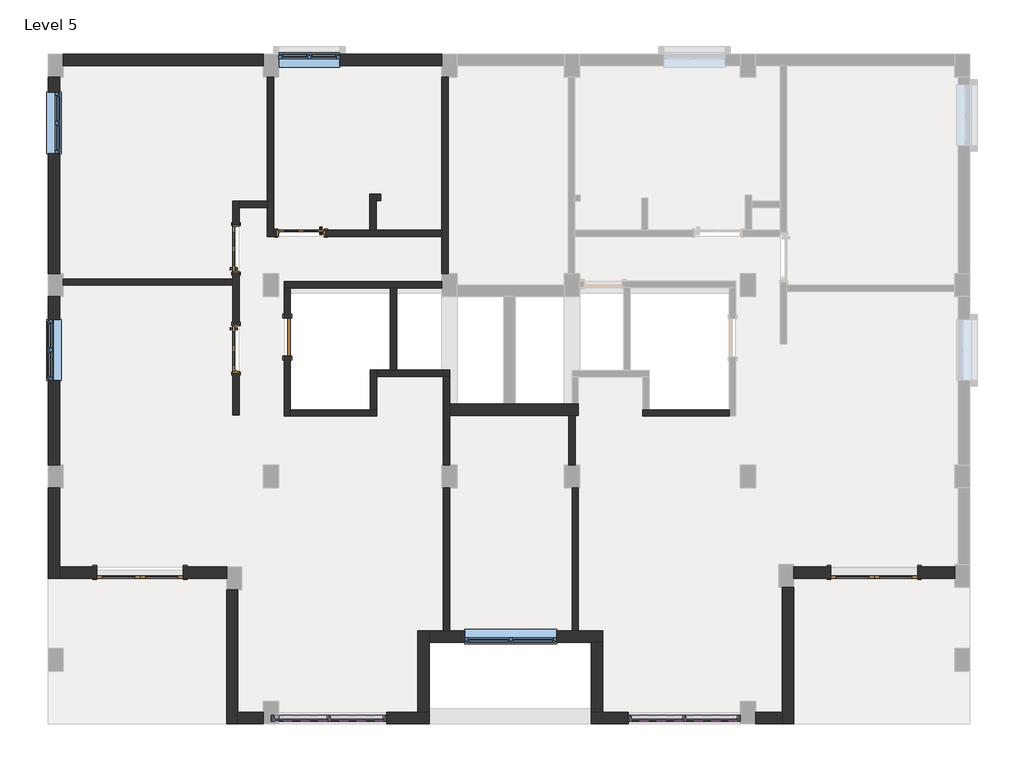
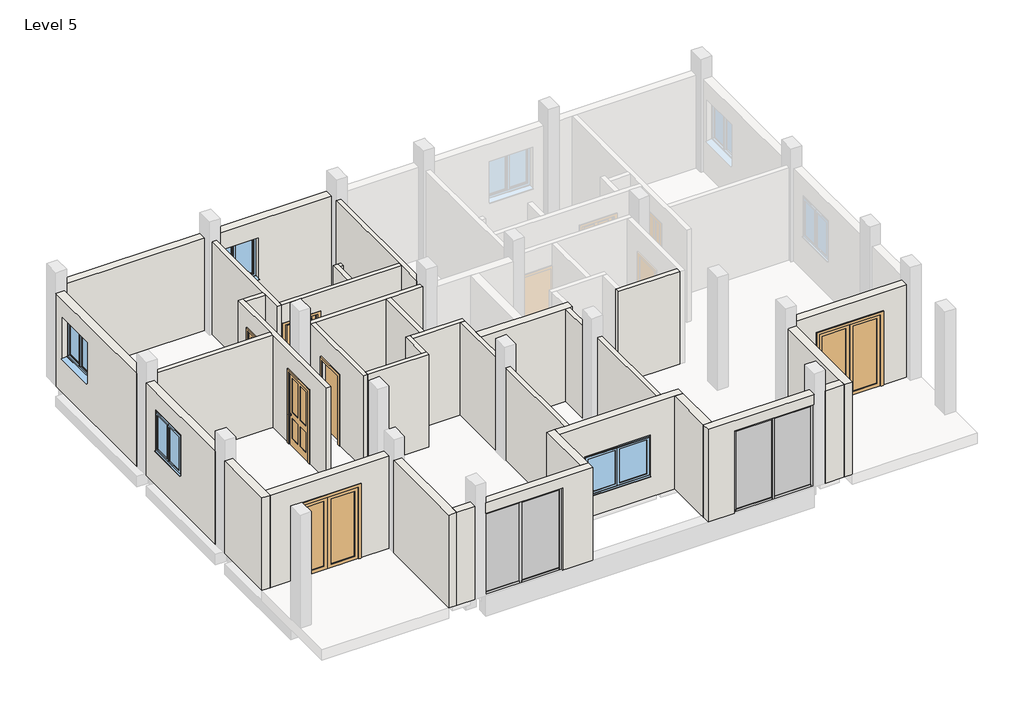
# One storey, part 1 of 3: 36 walls, 14 members, 6 doors, 4 plates, 4 windows.
"""IFC4 building model written with IfcOpenShell, lengths in millimetres."""

from ifc_helpers import new_model, si_unit, frame, origin, place, context, project, spatial, polyline, outline, extrude, faceted_brep, transform, mapped, element, save
from components import door_e52a3823, door_68a706ac, door_a823658d, door_1fe7f57d, member_a1c24a98, member_7fa39cca, member_f0fea5a5, member_ee409385, system_panel_glazed_8311221f, system_panel_glazed_a93c8db9, w2_0001_windows_4_x_4_9dec5fc7, w2_0001_window_4_x_6_83c3b52c

model = new_model("IFC4")

# Units and contexts
model_context = context("Model", 3, world=origin())
ifc_project = project(units=[si_unit("LENGTHUNIT", "METRE", prefix="MILLI")], contexts=[model_context])

# Site, building, storey
site = spatial("IfcSite", under=ifc_project)
building = spatial("IfcBuilding", under=site)
storey = spatial("IfcBuildingStorey", under=building, Name="Level 5", Elevation=6400.8)

# Doors
placement = place(None, origin())
door_shape = door_e52a3823(model_context)
element("IfcDoor", 1, ObjectType="Door-Double-Glass : 68\" x 84\"", at=placement, inside=storey, context=model_context, shape_type="MappedRepresentation", body=[
    mapped(door_shape, transform((-7309.9981098, -11554.5807833, 6400.8), x_axis=(-1.0, 0.0, 0.0), y_axis=(0.0, -1.0, 0.0), z_axis=(0.0, 0.0, 1.0))),
])
element("IfcDoor", 2, ObjectType="Door-Double-Glass : 68\" x 84\"", at=placement, inside=storey, context=model_context, shape_type="MappedRepresentation", body=[
    mapped(door_shape, transform((7313.6824202, -11554.5807833, 6400.8), x_axis=(-1.0, 0.0, 0.0), y_axis=(0.0, -1.0, 0.0), z_axis=(0.0, 0.0, 1.0))),
])
door_2_shape = door_68a706ac(model_context)
element("IfcDoor", 3, ObjectType="Door-Interior-Single-4_Panel-Wood : 36\" x 84\"", at=placement, inside=storey, context=model_context, shape_type="MappedRepresentation", body=[
    mapped(door_2_shape, transform((-5402.1925798, -5105.3620333, 6400.8), x_axis=(0.0, 1.0, 0.0), y_axis=(-1.0, 0.0, 0.0), z_axis=(0.0, 0.0, 1.0))),
])
door_3_shape = door_a823658d(model_context)
element("IfcDoor", 4, ObjectType="Door-Interior-Single-4_Panel-Wood : 36\" x 84\"", at=placement, inside=storey, context=model_context, shape_type="MappedRepresentation", body=[
    mapped(door_3_shape, transform((-4103.6175798, -4789.1311634, 6400.8), x_axis=(-1.0, 0.0, 0.0), y_axis=(0.0, -1.0, 0.0), z_axis=(0.0, 0.0, 1.0))),
])
element("IfcDoor", 5, ObjectType="Door-Interior-Single-4_Panel-Wood : 36\" x 84\"", at=placement, inside=storey, context=model_context, shape_type="MappedRepresentation", body=[
    mapped(door_3_shape, transform((-5402.1925798, -7092.9120333, 6400.8), x_axis=(0.0, -1.0, 0.0), y_axis=(1.0, 0.0, 0.0), z_axis=(0.0, 0.0, 1.0))),
])
door_4_shape = door_1fe7f57d(model_context)
element("IfcDoor", 6, ObjectType="Single-Flush : 30\" x 80\"", at=placement, inside=storey, context=model_context, shape_type="MappedRepresentation", body=[
    mapped(door_4_shape, transform((-4379.0950401, -6863.7942903, 6400.8), x_axis=(0.0, -1.0, 0.0), y_axis=(1.0, 0.0, 0.0), z_axis=(0.0, 0.0, 1.0))),
])

# Members
member_shape = member_a1c24a98(model_context)
element("IfcMember", 7, ObjectType="Rectangular Mullion : 2.5\" x 5\" rectangular", at=placement, inside=storey, context=model_context, shape_type="MappedRepresentation", body=[
    mapped(member_shape, transform((2474.9824202, -14462.5402089, 8839.2), x_axis=(0.0, 0.0, 1.0), y_axis=(0.0, 1.0, 0.0), z_axis=(-1.0, 0.0, 0.0))),
])
element("IfcMember", 8, ObjectType="Rectangular Mullion : 2.5\" x 5\" rectangular", at=placement, inside=storey, context=model_context, shape_type="MappedRepresentation", body=[
    mapped(member_shape, transform((3560.8324202, -14462.5402089, 8839.2), x_axis=(0.0, 0.0, 1.0), y_axis=(0.0, 1.0, 0.0), z_axis=(-1.0, 0.0, 0.0))),
])
element("IfcMember", 9, ObjectType="Rectangular Mullion : 2.5\" x 5\" rectangular", at=placement, inside=storey, context=model_context, shape_type="MappedRepresentation", body=[
    mapped(member_shape, transform((4583.1824202, -14462.5402089, 6400.8), x_axis=(0.0, 0.0, -1.0), y_axis=(0.0, 1.0, 0.0), z_axis=(1.0, 0.0, 0.0))),
])
element("IfcMember", 10, ObjectType="Rectangular Mullion : 2.5\" x 5\" rectangular", at=placement, inside=storey, context=model_context, shape_type="MappedRepresentation", body=[
    mapped(member_shape, transform((3497.3324202, -14462.5402089, 6400.8), x_axis=(0.0, 0.0, -1.0), y_axis=(0.0, 1.0, 0.0), z_axis=(1.0, 0.0, 0.0))),
])
member_2_shape = member_7fa39cca(model_context)
element("IfcMember", 11, ObjectType="Rectangular Mullion : 2.5\" x 5\" rectangular", at=placement, inside=storey, context=model_context, shape_type="MappedRepresentation", body=[
    mapped(member_2_shape, transform((-4637.0175798, -14462.5402089, 8839.2), x_axis=(0.0, 0.0, 1.0), y_axis=(0.0, 1.0, 0.0), z_axis=(-1.0, 0.0, 0.0))),
])
element("IfcMember", 12, ObjectType="Rectangular Mullion : 2.5\" x 5\" rectangular", at=placement, inside=storey, context=model_context, shape_type="MappedRepresentation", body=[
    mapped(member_2_shape, transform((-3519.4175798, -14462.5402089, 8839.2), x_axis=(0.0, 0.0, 1.0), y_axis=(0.0, 1.0, 0.0), z_axis=(-1.0, 0.0, 0.0))),
])
element("IfcMember", 13, ObjectType="Rectangular Mullion : 2.5\" x 5\" rectangular", at=placement, inside=storey, context=model_context, shape_type="MappedRepresentation", body=[
    mapped(member_2_shape, transform((-2465.3175798, -14462.5402089, 6400.8), x_axis=(0.0, 0.0, -1.0), y_axis=(0.0, 1.0, 0.0), z_axis=(1.0, 0.0, 0.0))),
])
element("IfcMember", 14, ObjectType="Rectangular Mullion : 2.5\" x 5\" rectangular", at=placement, inside=storey, context=model_context, shape_type="MappedRepresentation", body=[
    mapped(member_2_shape, transform((-3582.9175798, -14462.5402089, 6400.8), x_axis=(0.0, 0.0, -1.0), y_axis=(0.0, 1.0, 0.0), z_axis=(1.0, 0.0, 0.0))),
])
member_3_shape = member_f0fea5a5(model_context)
element("IfcMember", 15, ObjectType="Rectangular Mullion : 2.5\" x 5\" rectangular", at=placement, inside=storey, context=model_context, shape_type="MappedRepresentation", body=[
    mapped(member_3_shape, transform((3529.0824202, -14462.5402089, 6400.8), x_axis=(-1.0, 0.0, 0.0), y_axis=(0.0, 1.0, 0.0), z_axis=(0.0, 0.0, -1.0))),
])
element("IfcMember", 16, ObjectType="Rectangular Mullion : 2.5\" x 5\" rectangular", at=placement, inside=storey, context=model_context, shape_type="MappedRepresentation", body=[
    mapped(member_3_shape, transform((-3551.1675798, -14462.5402089, 6400.8), x_axis=(-1.0, 0.0, 0.0), y_axis=(0.0, 1.0, 0.0), z_axis=(0.0, 0.0, -1.0))),
])
member_4_shape = member_ee409385(model_context)
element("IfcMember", 17, ObjectType="Rectangular Mullion : 2.5\" x 5\" rectangular", at=placement, inside=storey, context=model_context, shape_type="MappedRepresentation", body=[
    mapped(member_4_shape, transform((2411.4824202, -14462.5402089, 6400.8), x_axis=(-1.0, 0.0, 0.0), y_axis=(0.0, 1.0, 0.0), z_axis=(0.0, 0.0, -1.0))),
])
element("IfcMember", 18, ObjectType="Rectangular Mullion : 2.5\" x 5\" rectangular", at=placement, inside=storey, context=model_context, shape_type="MappedRepresentation", body=[
    mapped(member_4_shape, transform((-4700.5175798, -14462.5402089, 6400.8), x_axis=(-1.0, 0.0, 0.0), y_axis=(0.0, 1.0, 0.0), z_axis=(0.0, 0.0, -1.0))),
])
element("IfcMember", 19, ObjectType="Rectangular Mullion : 2.5\" x 5\" rectangular", at=placement, inside=storey, context=model_context, shape_type="MappedRepresentation", body=[
    mapped(member_4_shape, transform((4646.6824202, -14462.5402089, 8839.2), x_axis=(1.0, 0.0, 0.0), y_axis=(0.0, 1.0, 0.0), z_axis=(0.0, 0.0, 1.0))),
])
element("IfcMember", 20, ObjectType="Rectangular Mullion : 2.5\" x 5\" rectangular", at=placement, inside=storey, context=model_context, shape_type="MappedRepresentation", body=[
    mapped(member_4_shape, transform((-2401.8175798, -14462.5402089, 8839.2), x_axis=(1.0, 0.0, 0.0), y_axis=(0.0, 1.0, 0.0), z_axis=(0.0, 0.0, 1.0))),
])

# Plates
system_panel_glazed_shape = system_panel_glazed_8311221f(model_context)
element("IfcPlate", 21, ObjectType="System Panel : Glazed", at=placement, inside=storey, context=model_context, shape_type="MappedRepresentation", body=[
    mapped(system_panel_glazed_shape, transform((4072.0074202, -14462.5402089, 6464.3), x_axis=(-1.0, 0.0, 0.0), y_axis=(0.0, -1.0, 0.0), z_axis=(0.0, 0.0, 1.0))),
])
element("IfcPlate", 22, ObjectType="System Panel : Glazed", at=placement, inside=storey, context=model_context, shape_type="MappedRepresentation", body=[
    mapped(system_panel_glazed_shape, transform((2986.1574202, -14462.5402089, 6464.3), x_axis=(-1.0, 0.0, 0.0), y_axis=(0.0, -1.0, 0.0), z_axis=(0.0, 0.0, 1.0))),
])
system_panel_glazed_2_shape = system_panel_glazed_a93c8db9(model_context)
element("IfcPlate", 23, ObjectType="System Panel : Glazed", at=placement, inside=storey, context=model_context, shape_type="MappedRepresentation", body=[
    mapped(system_panel_glazed_2_shape, transform((-2992.3675798, -14462.5402089, 6464.3), x_axis=(-1.0, 0.0, 0.0), y_axis=(0.0, -1.0, 0.0), z_axis=(0.0, 0.0, 1.0))),
])
element("IfcPlate", 24, ObjectType="System Panel : Glazed", at=placement, inside=storey, context=model_context, shape_type="MappedRepresentation", body=[
    mapped(system_panel_glazed_2_shape, transform((-4109.9675798, -14462.5402089, 6464.3), x_axis=(-1.0, 0.0, 0.0), y_axis=(0.0, -1.0, 0.0), z_axis=(0.0, 0.0, 1.0))),
])

# Walls
element("IfcWall", 25, ObjectType="EXTERIOR WALL 9\"", at=placement, inside=storey, context=model_context, shape_type="SweptSolid", body=[
    extrude(outline(polyline([(-4852.9175798, -1452.2061634), (-8839.9786397, -1452.2061634), (-8839.9786397, -1223.6061634), (-4852.9175798, -1223.6061634), (-4852.9175798, -1452.2061634)])), frame((0.0, 0.0, 6400.8), z_axis=(0.0, 0.0, 1.0), x_axis=(1.0, 0.0, 0.0)), (0.0, 0.0, 1.0), 2743.2),
])
element("IfcWall", 26, ObjectType="EXTERIOR WALL 9\"", at=placement, inside=storey, context=model_context, shape_type="SweptSolid", body=[
    extrude(outline(polyline([(7400.8, -3328.9175798), (7400.8, -4548.1175798), (6400.8, -4548.1175798), (6400.8, -1296.9175798), (9144.0, -1296.9175798), (9144.0, -4548.1175798), (8620.0, -4548.1175798), (8620.0, -3328.9175798), (7400.8, -3328.9175798)])), frame((0.0, -1452.2061634, 0.0), z_axis=(0.0, 1.0, 0.0), x_axis=(0.0, 0.0, 1.0)), (0.0, 0.0, 1.0), 228.6),
])
element("IfcWall", 27, ObjectType="EXTERIOR WALL 9\"", at=placement, inside=storey, context=model_context, shape_type="SweptSolid", body=[
    extrude(outline(polyline([(-1680.8061634, 6400.8), (-5600.6620333, 6400.8), (-5600.6620333, 9144.0), (-1680.8061634, 9144.0), (-1680.8061634, 6400.8)]), holes=[polyline([(-3204.8061634, 7400.8), (-1985.6061634, 7400.8), (-1985.6061634, 8620.0), (-3204.8061634, 8620.0), (-3204.8061634, 7400.8)])]), frame((-9144.7786397, 0.0, 0.0), z_axis=(1.0, 0.0, 0.0), x_axis=(0.0, 1.0, 0.0)), (0.0, 0.0, 1.0), 228.6),
])
element("IfcWall", 28, ObjectType="EXTERIOR WALL 9\"", at=placement, inside=storey, context=model_context, shape_type="SweptSolid", body=[
    extrude(outline(polyline([(-6057.8620333, 6400.8), (-9410.6620333, 6400.8), (-9410.6620333, 9144.0), (-6057.8620333, 9144.0), (-6057.8620333, 6400.8)]), holes=[polyline([(-6515.0620333, 7400.8), (-6515.0620333, 8620.0), (-7734.2620333, 8620.0), (-7734.2620333, 7400.8), (-6515.0620333, 7400.8)])]), frame((-9144.7786397, 0.0, 0.0), z_axis=(1.0, 0.0, 0.0), x_axis=(0.0, 1.0, 0.0)), (0.0, 0.0, 1.0), 228.6),
])
element("IfcWall", 29, ObjectType="EXTERIOR WALL 9\"", at=placement, inside=storey, context=model_context, shape_type="Brep", body=[
    faceted_brep([(-9144.7786397, -9867.8620333, 6400.8), (-9144.7786397, -11671.2620333, 6400.8), (-9144.7786397, -11671.2620333, 9144.0), (-9144.7786397, -9867.8620333, 9144.0), (-8916.1786397, -9867.8620333, 6400.8), (-8916.1786397, -9867.8620333, 9144.0), (-8916.1786397, -11442.6620333, 9144.0), (-8916.1786397, -11671.2620333, 9144.0), (-8916.1786397, -11671.2620333, 6400.8), (-8916.1786397, -11442.6620333, 6400.8)], [[[0, 1, 2, 3]], [[4, 5, 6, 7, 8, 9]], [[1, 0, 4, 9, 8]], [[3, 2, 7, 6, 5]], [[0, 3, 5, 4]], [[2, 1, 8, 7]]]),
])
element("IfcWall", 30, ObjectType="EXTERIOR WALL 9\"", at=placement, inside=storey, context=model_context, shape_type="SweptSolid", body=[
    extrude(outline(polyline([(9144.0, -5589.5175798), (9144.0, -8916.1786397), (6400.8, -8916.1786397), (6400.8, -8173.5981098), (8534.4, -8173.5981098), (8534.4, -6446.3981098), (6400.8, -6446.3981098), (6400.8, -5589.5175798), (9144.0, -5589.5175798)])), frame((0.0, -11671.2620333, 0.0), z_axis=(0.0, 1.0, 0.0), x_axis=(0.0, 0.0, 1.0)), (0.0, 0.0, 1.0), 228.6),
])
element("IfcWall", 31, ObjectType="EXTERIOR WALL 9\"", at=placement, inside=storey, context=model_context, shape_type="SweptSolid", body=[
    extrude(outline(polyline([(9144.0, 5713.4824202), (6400.8, 5713.4824202), (6400.8, 6450.0824202), (8534.4, 6450.0824202), (8534.4, 8177.2824202), (6400.8, 8177.2824202), (6400.8, 8913.8824202), (9144.0, 8913.8824202), (9144.0, 5713.4824202)])), frame((0.0, -11671.2620333, 0.0), z_axis=(0.0, 1.0, 0.0), x_axis=(0.0, 0.0, 1.0)), (0.0, 0.0, 1.0), 228.6),
])
element("IfcWall", 32, ObjectType="EXTERIOR WALL 9\"", at=placement, inside=storey, context=model_context, shape_type="Brep", body=[
    faceted_brep([(5484.8824202, -11849.0620333, 6400.8), (5484.8824202, -14348.2402089, 6400.8), (5484.8824202, -14576.8402089, 6400.8), (5484.8824202, -14576.8402089, 9144.0), (5484.8824202, -14348.2402089, 9144.0), (5484.8824202, -11849.0620333, 9144.0), (5713.4824202, -11849.0620333, 6400.8), (5713.4824202, -11849.0620333, 9144.0), (5713.4824202, -14576.8402089, 9144.0), (5713.4824202, -14576.8402089, 6400.8)], [[[0, 1, 2, 3, 4, 5]], [[6, 7, 8, 9]], [[2, 1, 0, 6, 9]], [[5, 4, 3, 8, 7]], [[0, 5, 7, 6]], [[3, 2, 9, 8]]]),
])
element("IfcWall", 33, ObjectType="EXTERIOR WALL 9\"", at=placement, inside=storey, context=model_context, shape_type="SweptSolid", body=[
    extrude(outline(polyline([(5484.8824202, -14576.8402089), (4951.4824202, -14576.8402089), (4951.4824202, -14348.2402089), (5484.8824202, -14348.2402089), (5484.8824202, -14576.8402089)])), frame((0.0, 0.0, 6400.8), z_axis=(0.0, 0.0, 1.0), x_axis=(1.0, 0.0, 0.0)), (0.0, 0.0, 1.0), 2743.2),
])
element("IfcWall", 34, ObjectType="EXTERIOR WALL 9\"", at=placement, inside=storey, context=model_context, shape_type="Brep", body=[
    faceted_brep([(-5589.5175798, -11899.8620333, 6400.8), (-5589.5175798, -14576.8402089, 6400.8), (-5589.5175798, -14576.8402089, 9144.0), (-5589.5175798, -11899.8620333, 9144.0), (-5360.9175798, -11899.8620333, 6400.8), (-5360.9175798, -11899.8620333, 9144.0), (-5360.9175798, -14348.2402089, 9144.0), (-5360.9175798, -14576.8402089, 9144.0), (-5360.9175798, -14576.8402089, 6400.8), (-5360.9175798, -14348.2402089, 6400.8)], [[[0, 1, 2, 3]], [[4, 5, 6, 7, 8, 9]], [[1, 0, 4, 9, 8]], [[3, 2, 7, 6, 5]], [[0, 3, 5, 4]], [[2, 1, 8, 7]]]),
])
element("IfcWall", 35, ObjectType="EXTERIOR WALL 9\"", at=placement, inside=storey, context=model_context, shape_type="SweptSolid", body=[
    extrude(outline(polyline([(-5360.9175798, -14348.2402089), (-4852.9175798, -14348.2402089), (-4852.9175798, -14576.8402089), (-5360.9175798, -14576.8402089), (-5360.9175798, -14348.2402089)])), frame((0.0, 0.0, 6400.8), z_axis=(0.0, 0.0, 1.0), x_axis=(1.0, 0.0, 0.0)), (0.0, 0.0, 1.0), 2743.2),
])
element("IfcWall", 36, ObjectType="EXTERIOR WALL 9\"", at=placement, inside=storey, context=model_context, shape_type="Brep", body=[
    faceted_brep([(1674.8824202, -14348.2402089, 9144.0), (1903.4824202, -14348.2402089, 9144.0), (4646.6824202, -14348.2402089, 9144.0), (4646.6824202, -14348.2402089, 8839.2), (2411.4824202, -14348.2402089, 8839.2), (2411.4824202, -14348.2402089, 6400.8), (1903.4824202, -14348.2402089, 6400.8), (1674.8824202, -14348.2402089, 6400.8), (4646.6824202, -14576.8402089, 9144.0), (1674.8824202, -14576.8402089, 9144.0), (1674.8824202, -14576.8402089, 6400.8), (2411.4824202, -14576.8402089, 6400.8), (2411.4824202, -14576.8402089, 8839.2), (4646.6824202, -14576.8402089, 8839.2)], [[[0, 1, 2, 3, 4, 5, 6, 7]], [[8, 9, 10, 11, 12, 13]], [[10, 7, 6, 5, 11]], [[2, 1, 0, 9, 8]], [[2, 8, 13, 3]], [[0, 7, 10, 9]], [[4, 12, 11, 5]], [[12, 4, 3, 13]]]),
])
element("IfcWall", 37, ObjectType="EXTERIOR WALL 9\"", at=placement, inside=storey, context=model_context, shape_type="Brep", body=[
    faceted_brep([(-1550.9175798, -14576.8402089, 9144.0), (-4548.1175798, -14576.8402089, 9144.0), (-4548.1175798, -14576.8402089, 8839.2), (-2401.8175798, -14576.8402089, 8839.2), (-2401.8175798, -14576.8402089, 6400.8), (-1550.9175798, -14576.8402089, 6400.8), (-4548.1175798, -14348.2402089, 9144.0), (-1779.5175798, -14348.2402089, 9144.0), (-1550.9175798, -14348.2402089, 9144.0), (-1550.9175798, -14348.2402089, 6400.8), (-1779.5175798, -14348.2402089, 6400.8), (-2401.8175798, -14348.2402089, 6400.8), (-2401.8175798, -14348.2402089, 8839.2), (-4548.1175798, -14348.2402089, 8839.2)], [[[0, 1, 2, 3, 4, 5]], [[6, 7, 8, 9, 10, 11, 12, 13]], [[9, 5, 4, 11, 10]], [[1, 0, 8, 7, 6]], [[1, 6, 13, 2]], [[0, 5, 9, 8]], [[3, 12, 11, 4]], [[12, 3, 2, 13]]]),
])
element("IfcWall", 38, ObjectType="EXTERIOR WALL 9\"", at=placement, inside=storey, context=model_context, shape_type="Brep", body=[
    faceted_brep([(-1550.9175798, -14348.2402089, 6400.8), (-1550.9175798, -12951.2402089, 6400.8), (-1550.9175798, -12722.6402089, 6400.8), (-1550.9175798, -12722.6402089, 9144.0), (-1550.9175798, -12951.2402089, 9144.0), (-1550.9175798, -14348.2402089, 9144.0), (-1779.5175798, -14348.2402089, 6400.8), (-1779.5175798, -14348.2402089, 9144.0), (-1779.5175798, -12722.6402089, 9144.0), (-1779.5175798, -12722.6402089, 6400.8)], [[[0, 1, 2, 3, 4, 5]], [[6, 7, 8, 9]], [[2, 1, 0, 6, 9]], [[5, 4, 3, 8, 7]], [[0, 5, 7, 6]], [[3, 2, 9, 8]]]),
])
element("IfcWall", 39, ObjectType="EXTERIOR WALL 9\"", at=placement, inside=storey, context=model_context, shape_type="Brep", body=[
    faceted_brep([(-1550.9175798, -12951.2402089, 6400.8), (1674.8824202, -12951.2402089, 6400.8), (1903.4824202, -12951.2402089, 6400.8), (1903.4824202, -12951.2402089, 9144.0), (1674.8824202, -12951.2402089, 9144.0), (-1550.9175798, -12951.2402089, 9144.0), (-839.7175798, -12951.2402089, 7010.4), (-839.7175798, -12951.2402089, 8229.6), (989.0824202, -12951.2402089, 8229.6), (989.0824202, -12951.2402089, 7010.4), (-1550.9175798, -12722.6402089, 6400.8), (-1550.9175798, -12722.6402089, 9144.0), (-1271.5175798, -12722.6402089, 9144.0), (-1144.5175798, -12722.6402089, 9144.0), (1293.8824202, -12722.6402089, 9144.0), (1420.8824202, -12722.6402089, 9144.0), (1903.4824202, -12722.6402089, 9144.0), (1903.4824202, -12722.6402089, 6400.8), (1420.8824202, -12722.6402089, 6400.8), (1293.8824202, -12722.6402089, 6400.8), (-1144.5175798, -12722.6402089, 6400.8), (-1271.5175798, -12722.6402089, 6400.8), (-839.7175798, -12722.6402089, 7010.4), (989.0824202, -12722.6402089, 7010.4), (989.0824202, -12722.6402089, 8229.6), (-839.7175798, -12722.6402089, 8229.6)], [[[0, 1, 2, 3, 4, 5], [6, 7, 8, 9]], [[10, 11, 12, 13, 14, 15, 16, 17, 18, 19, 20, 21], [22, 23, 24, 25]], [[2, 1, 0, 10, 21, 20, 19, 18, 17]], [[5, 4, 3, 16, 15, 14, 13, 12, 11]], [[0, 5, 11, 10]], [[3, 2, 17, 16]], [[7, 6, 22, 25]], [[8, 7, 25, 24]], [[9, 8, 24, 23]], [[6, 9, 23, 22]]]),
])
element("IfcWall", 40, ObjectType="EXTERIOR WALL 9\"", at=placement, inside=storey, context=model_context, shape_type="SweptSolid", body=[
    extrude(outline(polyline([(1674.8824202, -14348.2402089), (1674.8824202, -12951.2402089), (1903.4824202, -12951.2402089), (1903.4824202, -14348.2402089), (1674.8824202, -14348.2402089)])), frame((0.0, 0.0, 6400.8), z_axis=(0.0, 0.0, 1.0), x_axis=(1.0, 0.0, 0.0)), (0.0, 0.0, 1.0), 2743.2),
])
element("IfcWall", 41, ObjectType="EXTERIOR WALL 9\"", at=placement, inside=storey, context=model_context, shape_type="Brep", body=[
    faceted_brep([(-1144.5175798, -8426.4120333, 6400.8), (1230.3824202, -8426.4120333, 6400.8), (1357.3824202, -8426.4120333, 6400.8), (1420.8824202, -8426.4120333, 6400.8), (1420.8824202, -8426.4120333, 9144.0), (1357.3824202, -8426.4120333, 9144.0), (1230.3824202, -8426.4120333, 9144.0), (-1144.5175798, -8426.4120333, 9144.0), (-1144.5175798, -8197.8120333, 6400.8), (-1144.5175798, -8197.8120333, 9144.0), (-65.0175798, -8197.8120333, 9144.0), (163.5824202, -8197.8120333, 9144.0), (1293.8824202, -8197.8120333, 9144.0), (1420.8824202, -8197.8120333, 9144.0), (1420.8824202, -8197.8120333, 6400.8), (1293.8824202, -8197.8120333, 6400.8), (163.5824202, -8197.8120333, 6400.8), (-65.0175798, -8197.8120333, 6400.8)], [[[0, 1, 2, 3, 4, 5, 6, 7]], [[8, 9, 10, 11, 12, 13, 14, 15, 16, 17]], [[3, 2, 1, 0, 8, 17, 16, 15, 14]], [[7, 6, 5, 4, 13, 12, 11, 10, 9]], [[0, 7, 9, 8]], [[4, 3, 14, 13]]]),
])
element("IfcWall", 42, ObjectType="INTERIOR WALL 5\"", at=placement, inside=storey, context=model_context, shape_type="SweptSolid", body=[
    extrude(outline(polyline([(-5462.5175798, -5829.2620333), (-8839.9786397, -5829.2620333), (-8839.9786397, -5702.2620333), (-5462.5175798, -5702.2620333), (-5462.5175798, -5829.2620333)])), frame((0.0, 0.0, 6400.8), z_axis=(0.0, 0.0, 1.0), x_axis=(1.0, 0.0, 0.0)), (0.0, 0.0, 1.0), 2743.2),
])
element("IfcWall", 43, ObjectType="INTERIOR WALL 5\"", at=placement, inside=storey, context=model_context, shape_type="Brep", body=[
    faceted_brep([(-5462.5175798, -8420.0620333, 6400.8), (-5462.5175798, -8420.0620333, 9144.0), (-5462.5175798, -5829.2620333, 9144.0), (-5462.5175798, -5702.2620333, 9144.0), (-5462.5175798, -4153.3104011, 9144.0), (-5462.5175798, -4153.3104011, 6400.8), (-5462.5175798, -4622.7620333, 6400.8), (-5462.5175798, -4622.7620333, 8559.8), (-5462.5175798, -5587.9620333, 8559.8), (-5462.5175798, -5587.9620333, 6400.8), (-5462.5175798, -5702.2620333, 6400.8), (-5462.5175798, -5829.2620333, 6400.8), (-5462.5175798, -6610.3120333, 6400.8), (-5462.5175798, -6610.3120333, 8559.8), (-5462.5175798, -7575.5120333, 8559.8), (-5462.5175798, -7575.5120333, 6400.8), (-5335.5175798, -8420.0620333, 9144.0), (-5335.5175798, -8420.0620333, 6400.8), (-5335.5175798, -7575.5120333, 6400.8), (-5335.5175798, -7575.5120333, 8559.8), (-5335.5175798, -6610.3120333, 8559.8), (-5335.5175798, -6610.3120333, 6400.8), (-5335.5175798, -5587.9620333, 6400.8), (-5335.5175798, -5587.9620333, 8559.8), (-5335.5175798, -4622.7620333, 8559.8), (-5335.5175798, -4622.7620333, 6400.8), (-5335.5175798, -4280.3104011, 6400.8), (-5335.5175798, -4153.3104011, 6400.8), (-5335.5175798, -4153.3104011, 9144.0), (-5335.5175798, -4280.3104011, 9144.0)], [[[0, 1, 2, 3, 4, 5, 6, 7, 8, 9, 10, 11, 12, 13, 14, 15]], [[16, 17, 18, 19, 20, 21, 22, 23, 24, 25, 26, 27, 28, 29]], [[17, 0, 15, 18]], [[5, 27, 26, 25, 6]], [[9, 22, 21, 12, 11, 10]], [[1, 0, 17, 16]], [[4, 3, 2, 1, 16, 29, 28]], [[5, 4, 28, 27]], [[24, 7, 6, 25]], [[7, 24, 23, 8]], [[8, 23, 22, 9]], [[14, 19, 18, 15]], [[19, 14, 13, 20]], [[20, 13, 12, 21]]]),
])
element("IfcWall", 44, ObjectType="INTERIOR WALL 5\"", at=placement, inside=storey, context=model_context, shape_type="SweptSolid", body=[
    extrude(outline(polyline([(-4776.7175798, -4280.3104011), (-5335.5175798, -4280.3104011), (-5335.5175798, -4153.3104011), (-4776.7175798, -4153.3104011), (-4776.7175798, -4280.3104011)])), frame((0.0, 0.0, 6400.8), z_axis=(0.0, 0.0, 1.0), x_axis=(1.0, 0.0, 0.0)), (0.0, 0.0, 1.0), 2743.2),
])
element("IfcWall", 45, ObjectType="INTERIOR WALL 5\"", at=placement, inside=storey, context=model_context, shape_type="Brep", body=[
    faceted_brep([(-4776.7175798, -1680.8061634, 6400.8), (-4776.7175798, -4153.3104011, 6400.8), (-4776.7175798, -4280.3104011, 6400.8), (-4776.7175798, -4855.8061634, 6400.8), (-4776.7175798, -4855.8061634, 9144.0), (-4776.7175798, -4280.3104011, 9144.0), (-4776.7175798, -4153.3104011, 9144.0), (-4776.7175798, -1680.8061634, 9144.0), (-4649.7175798, -1680.8061634, 6400.8), (-4649.7175798, -1680.8061634, 9144.0), (-4649.7175798, -4728.8061634, 9144.0), (-4649.7175798, -4855.8061634, 9144.0), (-4649.7175798, -4855.8061634, 6400.8), (-4649.7175798, -4728.8061634, 6400.8)], [[[0, 1, 2, 3, 4, 5, 6, 7]], [[8, 9, 10, 11, 12, 13]], [[3, 2, 1, 0, 8, 13, 12]], [[7, 6, 5, 4, 11, 10, 9]], [[0, 7, 9, 8]], [[4, 3, 12, 11]]]),
])
element("IfcWall", 46, ObjectType="INTERIOR WALL 5\"", at=placement, inside=storey, context=model_context, shape_type="Brep", body=[
    faceted_brep([(-1296.9175798, -4855.8061634, 9144.0), (-4649.7175798, -4855.8061634, 9144.0), (-4649.7175798, -4855.8061634, 6400.8), (-4586.2175798, -4855.8061634, 6400.8), (-4586.2175798, -4855.8061634, 8559.8), (-3621.0175798, -4855.8061634, 8559.8), (-3621.0175798, -4855.8061634, 6400.8), (-1296.9175798, -4855.8061634, 6400.8), (-4649.7175798, -4728.8061634, 9144.0), (-2732.0175798, -4728.8061634, 9144.0), (-2605.0175798, -4728.8061634, 9144.0), (-1296.9175798, -4728.8061634, 9144.0), (-1296.9175798, -4728.8061634, 6400.8), (-2605.0175798, -4728.8061634, 6400.8), (-2732.0175798, -4728.8061634, 6400.8), (-3621.0175798, -4728.8061634, 6400.8), (-3621.0175798, -4728.8061634, 8559.8), (-4586.2175798, -4728.8061634, 8559.8), (-4586.2175798, -4728.8061634, 6400.8), (-4649.7175798, -4728.8061634, 6400.8)], [[[0, 1, 2, 3, 4, 5, 6, 7]], [[8, 9, 10, 11, 12, 13, 14, 15, 16, 17, 18, 19]], [[2, 19, 18, 3]], [[12, 7, 6, 15, 14, 13]], [[1, 0, 11, 10, 9, 8]], [[2, 1, 8, 19]], [[0, 7, 12, 11]], [[17, 4, 3, 18]], [[4, 17, 16, 5]], [[5, 16, 15, 6]]]),
])
element("IfcWall", 47, ObjectType="INTERIOR WALL 5\"", at=placement, inside=storey, context=model_context, shape_type="Brep", body=[
    faceted_brep([(-1296.9175798, -1680.8061634, 6400.8), (-1296.9175798, -4728.8061634, 6400.8), (-1296.9175798, -4855.8061634, 6400.8), (-1296.9175798, -5600.6620333, 6400.8), (-1296.9175798, -5600.6620333, 9144.0), (-1296.9175798, -4855.8061634, 9144.0), (-1296.9175798, -4728.8061634, 9144.0), (-1296.9175798, -1680.8061634, 9144.0), (-1169.9175798, -1680.8061634, 6400.8), (-1169.9175798, -1680.8061634, 9144.0), (-1169.9175798, -5600.6620333, 9144.0), (-1169.9175798, -5600.6620333, 6400.8)], [[[0, 1, 2, 3, 4, 5, 6, 7]], [[8, 9, 10, 11]], [[3, 2, 1, 0, 8, 11]], [[4, 3, 11, 10]], [[7, 6, 5, 4, 10, 9]], [[0, 7, 9, 8]]]),
])
element("IfcWall", 48, ObjectType="INTERIOR WALL 5\"", at=placement, inside=storey, context=model_context, shape_type="Brep", body=[
    faceted_brep([(-2605.0175798, -4728.8061634, 6400.8), (-2605.0175798, -4144.6061634, 6400.8), (-2605.0175798, -4017.6061634, 6400.8), (-2605.0175798, -4017.6061634, 9144.0), (-2605.0175798, -4144.6061634, 9144.0), (-2605.0175798, -4728.8061634, 9144.0), (-2732.0175798, -4728.8061634, 6400.8), (-2732.0175798, -4728.8061634, 9144.0), (-2732.0175798, -4017.6061634, 9144.0), (-2732.0175798, -4017.6061634, 6400.8)], [[[0, 1, 2, 3, 4, 5]], [[6, 7, 8, 9]], [[2, 1, 0, 6, 9]], [[5, 4, 3, 8, 7]], [[0, 5, 7, 6]], [[3, 2, 9, 8]]]),
])
element("IfcWall", 49, ObjectType="INTERIOR WALL 5\"", at=placement, inside=storey, context=model_context, shape_type="SweptSolid", body=[
    extrude(outline(polyline([(-2605.0175798, -4017.6061634), (-2516.1175798, -4017.6061634), (-2516.1175798, -4144.6061634), (-2605.0175798, -4144.6061634), (-2605.0175798, -4017.6061634)])), frame((0.0, 0.0, 6400.8), z_axis=(0.0, 0.0, 1.0), x_axis=(1.0, 0.0, 0.0)), (0.0, 0.0, 1.0), 2743.2),
])
element("IfcWall", 50, ObjectType="INTERIOR WALL 5\"", at=placement, inside=storey, context=model_context, shape_type="Brep", body=[
    faceted_brep([(-4442.5950401, -5885.8942903, 6400.8), (-4315.5950401, -5885.8942903, 6400.8), (-2325.6175798, -5885.8942903, 6400.8), (-2198.6175798, -5885.8942903, 6400.8), (-1296.9175798, -5885.8942903, 6400.8), (-1296.9175798, -5885.8942903, 9144.0), (-2198.6175798, -5885.8942903, 9144.0), (-2325.6175798, -5885.8942903, 9144.0), (-4315.5950401, -5885.8942903, 9144.0), (-4442.5950401, -5885.8942903, 9144.0), (-4442.5950401, -5758.8942903, 6400.8), (-4442.5950401, -5758.8942903, 9144.0), (-1296.9175798, -5758.8942903, 9144.0), (-1296.9175798, -5758.8942903, 6400.8)], [[[0, 1, 2, 3, 4, 5, 6, 7, 8, 9]], [[10, 11, 12, 13]], [[4, 3, 2, 1, 0, 10, 13]], [[5, 4, 13, 12]], [[9, 8, 7, 6, 5, 12, 11]], [[0, 9, 11, 10]]]),
])
element("IfcWall", 51, ObjectType="INTERIOR WALL 5\"", at=placement, inside=storey, context=model_context, shape_type="Brep", body=[
    faceted_brep([(-4442.5950401, -7244.7942903, 8432.8), (-4442.5950401, -7244.7942903, 6400.8), (-4442.5950401, -8439.1120333, 6400.8), (-4442.5950401, -8439.1120333, 9144.0), (-4442.5950401, -5885.8942903, 9144.0), (-4442.5950401, -5885.8942903, 6400.8), (-4442.5950401, -6482.7942903, 6400.8), (-4442.5950401, -6482.7942903, 8432.8), (-4315.5950401, -8439.1120333, 6400.8), (-4315.5950401, -8312.1120333, 6400.8), (-4315.5950401, -7244.7942903, 6400.8), (-4315.5950401, -7244.7942903, 8432.8), (-4315.5950401, -6482.7942903, 8432.8), (-4315.5950401, -6482.7942903, 6400.8), (-4315.5950401, -5885.8942903, 6400.8), (-4315.5950401, -5885.8942903, 9144.0), (-4315.5950401, -8312.1120333, 9144.0), (-4315.5950401, -8439.1120333, 9144.0)], [[[0, 1, 2, 3, 4, 5, 6, 7]], [[8, 9, 10, 11, 12, 13, 14, 15, 16, 17]], [[6, 5, 14, 13]], [[2, 1, 10, 9, 8]], [[4, 3, 17, 16, 15]], [[5, 4, 15, 14]], [[3, 2, 8, 17]], [[11, 10, 1, 0]], [[12, 11, 0, 7]], [[13, 12, 7, 6]]]),
])
element("IfcWall", 52, ObjectType="INTERIOR WALL 5\"", at=placement, inside=storey, context=model_context, shape_type="Brep", body=[
    faceted_brep([(-4315.5950401, -8439.1120333, 6400.8), (-2601.0950401, -8439.1120333, 6400.8), (-2601.0950401, -8439.1120333, 9144.0), (-4315.5950401, -8439.1120333, 9144.0), (-4315.5950401, -8312.1120333, 6400.8), (-4315.5950401, -8312.1120333, 9144.0), (-2728.0950401, -8312.1120333, 9144.0), (-2601.0950401, -8312.1120333, 9144.0), (-2601.0950401, -8312.1120333, 6400.8), (-2728.0950401, -8312.1120333, 6400.8)], [[[0, 1, 2, 3]], [[4, 5, 6, 7, 8, 9]], [[1, 0, 4, 9, 8]], [[3, 2, 7, 6, 5]], [[0, 3, 5, 4]], [[2, 1, 8, 7]]]),
])
element("IfcWall", 53, ObjectType="INTERIOR WALL 5\"", at=placement, inside=storey, context=model_context, shape_type="Brep", body=[
    faceted_brep([(-2601.0950401, -8312.1120333, 6400.8), (-2601.0950401, -7651.7120333, 6400.8), (-2601.0950401, -7524.7120333, 6400.8), (-2601.0950401, -7524.7120333, 9144.0), (-2601.0950401, -7651.7120333, 9144.0), (-2601.0950401, -8312.1120333, 9144.0), (-2728.0950401, -8312.1120333, 6400.8), (-2728.0950401, -8312.1120333, 9144.0), (-2728.0950401, -7524.7120333, 9144.0), (-2728.0950401, -7524.7120333, 6400.8)], [[[0, 1, 2, 3, 4, 5]], [[6, 7, 8, 9]], [[2, 1, 0, 6, 9]], [[5, 4, 3, 8, 7]], [[0, 5, 7, 6]], [[3, 2, 9, 8]]]),
])
element("IfcWall", 54, ObjectType="INTERIOR WALL 5\"", at=placement, inside=storey, context=model_context, shape_type="Brep", body=[
    faceted_brep([(-2601.0950401, -7651.7120333, 6400.8), (-1271.5175798, -7651.7120333, 6400.8), (-1144.5175798, -7651.7120333, 6400.8), (-1144.5175798, -7651.7120333, 9144.0), (-1271.5175798, -7651.7120333, 9144.0), (-2601.0950401, -7651.7120333, 9144.0), (-2601.0950401, -7524.7120333, 6400.8), (-2601.0950401, -7524.7120333, 9144.0), (-2325.6175798, -7524.7120333, 9144.0), (-2198.6175798, -7524.7120333, 9144.0), (-1144.5175798, -7524.7120333, 9144.0), (-1144.5175798, -7524.7120333, 6400.8), (-2198.6175798, -7524.7120333, 6400.8), (-2325.6175798, -7524.7120333, 6400.8)], [[[0, 1, 2, 3, 4, 5]], [[6, 7, 8, 9, 10, 11, 12, 13]], [[2, 1, 0, 6, 13, 12, 11]], [[5, 4, 3, 10, 9, 8, 7]], [[0, 5, 7, 6]], [[3, 2, 11, 10]]]),
])
element("IfcWall", 55, ObjectType="INTERIOR WALL 5\"", at=placement, inside=storey, context=model_context, shape_type="SweptSolid", body=[
    extrude(outline(polyline([(-2325.6175798, -7524.7120333), (-2325.6175798, -5885.8942903), (-2198.6175798, -5885.8942903), (-2198.6175798, -7524.7120333), (-2325.6175798, -7524.7120333)])), frame((0.0, 0.0, 6400.8), z_axis=(0.0, 0.0, 1.0), x_axis=(1.0, 0.0, 0.0)), (0.0, 0.0, 1.0), 2743.2),
])
element("IfcWall", 56, ObjectType="INTERIOR WALL 5\"", at=placement, inside=storey, context=model_context, shape_type="Brep", body=[
    faceted_brep([(-1271.5175798, -7651.7120333, 6400.8), (-1271.5175798, -9417.0120333, 6400.8), (-1271.5175798, -9417.0120333, 9144.0), (-1271.5175798, -7651.7120333, 9144.0), (-1144.5175798, -7651.7120333, 6400.8), (-1144.5175798, -7651.7120333, 9144.0), (-1144.5175798, -8197.8120333, 9144.0), (-1144.5175798, -8426.4120333, 9144.0), (-1144.5175798, -9417.0120333, 9144.0), (-1144.5175798, -9417.0120333, 6400.8), (-1144.5175798, -8426.4120333, 6400.8), (-1144.5175798, -8197.8120333, 6400.8)], [[[0, 1, 2, 3]], [[4, 5, 6, 7, 8, 9, 10, 11]], [[1, 0, 4, 11, 10, 9]], [[2, 1, 9, 8]], [[3, 2, 8, 7, 6, 5]], [[0, 3, 5, 4]]]),
])
element("IfcWall", 57, ObjectType="INTERIOR WALL 5\"", at=placement, inside=storey, context=model_context, shape_type="Brep", body=[
    faceted_brep([(4430.7824202, -8312.7691591, 6400.8), (2830.5824202, -8312.7691591, 6400.8), (2703.5824202, -8312.7691591, 6400.8), (2703.5824202, -8312.7691591, 9144.0), (2830.5824202, -8312.7691591, 9144.0), (4430.7824202, -8312.7691591, 9144.0), (4430.7824202, -8439.7691591, 6400.8), (4430.7824202, -8439.7691591, 9144.0), (2703.5824202, -8439.7691591, 9144.0), (2703.5824202, -8439.7691591, 6400.8)], [[[0, 1, 2, 3, 4, 5]], [[6, 7, 8, 9]], [[2, 1, 0, 6, 9]], [[5, 4, 3, 8, 7]], [[0, 5, 7, 6]], [[3, 2, 9, 8]]]),
])
element("IfcWall", 58, ObjectType="INTERIOR WALL 5\"", at=placement, inside=storey, context=model_context, shape_type="SweptSolid", body=[
    extrude(outline(polyline([(-1271.5175798, -12722.6402089), (-1271.5175798, -9867.8620333), (-1144.5175798, -9867.8620333), (-1144.5175798, -12722.6402089), (-1271.5175798, -12722.6402089)])), frame((0.0, 0.0, 6400.8), z_axis=(0.0, 0.0, 1.0), x_axis=(1.0, 0.0, 0.0)), (0.0, 0.0, 1.0), 2743.2),
])
element("IfcWall", 59, ObjectType="INTERIOR WALL 5\"", at=placement, inside=storey, context=model_context, shape_type="SweptSolid", body=[
    extrude(outline(polyline([(1293.8824202, -12722.6402089), (1293.8824202, -9867.8620333), (1420.8824202, -9867.8620333), (1420.8824202, -12722.6402089), (1293.8824202, -12722.6402089)])), frame((0.0, 0.0, 6400.8), z_axis=(0.0, 0.0, 1.0), x_axis=(1.0, 0.0, 0.0)), (0.0, 0.0, 1.0), 2743.2),
])
element("IfcWall", 60, ObjectType="INTERIOR WALL 5\"", at=placement, inside=storey, context=model_context, shape_type="SweptSolid", body=[
    extrude(outline(polyline([(1357.3824202, -8426.4120333), (1357.3824202, -9410.6620333), (1230.3824202, -9410.6620333), (1230.3824202, -8426.4120333), (1357.3824202, -8426.4120333)])), frame((0.0, 0.0, 6400.8), z_axis=(0.0, 0.0, 1.0), x_axis=(1.0, 0.0, 0.0)), (0.0, 0.0, 1.0), 2743.2),
])

# Windows
w2_0001_windows_4_x_4_shape = w2_0001_windows_4_x_4_9dec5fc7(model_context)
element("IfcWindow", 61, ObjectType="w2.0001 : WINDOWS 4' X 4'", at=placement, inside=storey, context=model_context, shape_type="MappedRepresentation", body=[
    mapped(w2_0001_windows_4_x_4_shape, transform((-9030.4786397, -2595.2061634, 6400.8), x_axis=(0.0, 1.0, 0.0), y_axis=(-1.0, 0.0, 0.0), z_axis=(0.0, 0.0, 1.0))),
])
element("IfcWindow", 62, ObjectType="w2.0001 : WINDOWS 4' X 4'", at=placement, inside=storey, context=model_context, shape_type="MappedRepresentation", body=[
    mapped(w2_0001_windows_4_x_4_shape, transform((-9030.4786397, -7124.6620333, 6400.8), x_axis=(0.0, -1.0, 0.0), y_axis=(1.0, 0.0, 0.0), z_axis=(0.0, 0.0, 1.0))),
])
element("IfcWindow", 63, ObjectType="w2.0001 : WINDOWS 4' X 4'", at=placement, inside=storey, context=model_context, shape_type="MappedRepresentation", body=[
    mapped(w2_0001_windows_4_x_4_shape, transform((-3938.5175798, -1337.9061634, 6400.8), x_axis=(-1.0, 0.0, 0.0), y_axis=(0.0, -1.0, 0.0), z_axis=(0.0, 0.0, 1.0))),
])
w2_0001_window_4_x_6_shape = w2_0001_window_4_x_6_83c3b52c(model_context)
element("IfcWindow", 64, ObjectType="w2.0001 : window 4' x 6'", at=placement, inside=storey, context=model_context, shape_type="MappedRepresentation", body=[
    mapped(w2_0001_window_4_x_6_shape, transform((74.6824202, -12836.9402089, 6010.4), x_axis=(1.0, 0.0, 0.0), y_axis=(0.0, 1.0, 0.0), z_axis=(0.0, 0.0, 1.0))),
])

save(model, "model.ifc")

# Revit data of these elements
# Type "Door-Double-Glass : 68\" x 84\""
#   Type Mark = "11"
#   Construction Type Id = "opn-d45"
#   Assembly Code = "C1020"
#   Analytic Construction = "Wood frame, double glass door "
#   W = 2' - 10"
#   Thickness = 0' - 2"
#   Thermal Resistance (R) = 1.8150 (h·ft²·°F)/BTU
#   Swing Angle [instance default] = 90.00°
#   Heat Transfer Coefficient (U) = 0.5510 BTU/(h·ft²·°F)
#   Height = 7' - 0"
#   Bottom Rail = 0' - 4"
#   Top Rail = 0' - 4"
#   Stiles = 0' - 4"
#   Trim Projection = 0' - 1"
#   Trim Width = 0' - 3"
#   Width = 5' - 8"
#   Define Thermal Properties by = 1
#   Glazing = Glass
#   Panel Material = Wood - Birch - Solid Stained Light Low Gloss
#   Trim Material = Paint - Sienna
#   Visual Light Transmittance = 0
#   Solar Heat Gain Coefficient = 0
#   Function = (empty or 0)
#   Wall Closure = (empty or 0)
# Type "Door-Interior-Single-4_Panel-Wood : 36\" x 84\""
#   Type Mark = "9"
#   Assembly Code = "C1020300"
#   Analytic Construction = "Wooden"
#   Top Rail = 0' - 4 11/16"
#   Thickness = 0' - 1 3/8"
#   Thermal Resistance (R) = 2.5876 (h·ft²·°F)/BTU
#   Swing Angle [instance default] = 90.00°
#   Stiles = 0' - 4 3/4"
#   Rough Width = 3' - 2"
#   Rough Height = 7' - 1"
#   Mullion = 0' - 4 1/2"
#   Lock Rail = 0' - 7 1/2"
#   Height = 7' - 0"
#   Width = 3' - 0"
#   Heat Transfer Coefficient (U) = 0.3865 BTU/(h·ft²·°F)
#   Bottom Rail = 0' - 9 1/8"
#   Trim Material = Cherry
#   Panel Material = Cherry
#   Frame Material = Cherry
#   Door Handle Material = Aluminum
#   Visual Light Transmittance = 0
#   Solar Heat Gain Coefficient = 0
#   Wall Closure = (empty or 0)
#   Function = (empty or 0)
# Type "Single-Flush : 30\" x 80\""
#   Type Mark = "5"
#   Construction Type Id = "MDOOR"
#   Assembly Code = "C1020"
#   Analytic Construction = "Metal"
#   Thickness = 0' - 2"
#   Heat Transfer Coefficient (U) = 0.651978 BTU/(h·ft²·°F)
#   Height = 6' - 8"
#   Trim Projection Ext = 0' - 1"
#   Trim Projection Int = 0' - 1"
#   Trim Width = 0' - 3"
#   Width = 2' - 6"
#   Define Thermal Properties by = 1
#   Define Thermal Properties by = 1
#   Door Material = Door - Panel
#   Frame Material = Door - Frame
#   Visual Light Transmittance = 0
#   Solar Heat Gain Coefficient = 0
#   Function = (empty or 0)
#   Wall Closure = (empty or 0)
# Type "Rectangular Mullion : 2.5\" x 5\" rectangular"
#   built-in parameter 1007304 = 0.416667 (stored number, unit not read)
#   built-in parameter 1007301 = 0.104167 (stored number, unit not read)
#   built-in parameter 1007300 = 0.104167 (stored number, unit not read)
# Type "System Panel : Glazed"
#   Construction Type Id = "GSP4R"
#   Analytic Construction = "1/8 in Pilkington single glazing"
#   Visual Light Transmittance = 0.9
#   Solar Heat Gain Coefficient = 0.86
#   Heat Transfer Coefficient (U) = 1.18115 BTU/(h·ft²·°F)
#   Define Thermal Properties by = 1
# Type "EXTERIOR WALL 9\""
#   Assembly Code = "B2010"
#   Layers, outside or top first: 0' - 9" "WARM BEIGE COLOUR" (function 1)
# Type "INTERIOR WALL 5\""
#   Assembly Code = "B2010"
#   Layers, outside or top first: 0' - 5" "WARM BEIGE COLOUR" (function 1)
# Type "w2.0001 : WINDOWS 4' X 4'"
#   Type Mark = "21"
#   Operation = "DoublePanelVertical"
#   Keynote = "16.05.01"
#   Analytic Construction = "<None>"
#   Rough Width = 4' - 0"
#   Rough Height = 4' - 0"
#   Rahmentiefe = 0' - 2.3622"
#   Rahmenhöhe unten = 0' - 3.14961"
#   Rahmehöhe oben = 0' - 3.14961"
#   Rahmenbreite = 0' - 2.3622"
#   Height = 4' - 0"
#   Flügeltiefe = 0' - 2.3622"
#   Flügelbreite = 0' - 2.3622"
#   Einbautiefe (von außen) [instance default] = 0' - 5.51181"
#   Width = 4' - 0"
#   Kippflügel [instance default] = yes
#   Drehflügel im Grundriß darstellen [instance default] = no
#   Drehflügel [instance default] = yes
#   Define Thermal Properties by = 1
#   Rahmen [instance default] = none
#   Glas [instance default] = none
#   Flügel [instance default] = none
#   Fensterbank aussen [instance default] = none
#   Fensterbank innen [instance default] = none
#   Wall Closure = (empty or 0)
# Type "w2.0001 : window 4' x 6'"
#   Type Mark = "22"
#   Operation = "DoublePanelVertical"
#   Keynote = "16.05.01"
#   Analytic Construction = "<None>"
#   Rough Width = 6' - 0"
#   Rough Height = 4' - 0"
#   Rahmentiefe = 0' - 2.3622"
#   Rahmenhöhe unten = 0' - 3.14961"
#   Rahmehöhe oben = 0' - 3.14961"
#   Rahmenbreite = 0' - 2.3622"
#   Height = 4' - 0"
#   Flügeltiefe = 0' - 2.3622"
#   Flügelbreite = 0' - 2.3622"
#   Einbautiefe (von außen) [instance default] = 0' - 5.51181"
#   Width = 6' - 0"
#   Kippflügel [instance default] = yes
#   Drehflügel im Grundriß darstellen [instance default] = no
#   Drehflügel [instance default] = yes
#   Define Thermal Properties by = 1
#   Rahmen [instance default] = none
#   Glas [instance default] = none
#   Flügel [instance default] = none
#   Fensterbank aussen [instance default] = none
#   Fensterbank innen [instance default] = none
#   Wall Closure = (empty or 0)
# Elements 1, 2 (IfcDoor, "Door-Double-Glass : 68\" x 84\"")
#   Phase Created = New Construction
#   Materials on its faces: "Wood - Birch - Solid Stained Light Low Gloss", "Paint - Sienna", "Glass"
# Elements 3, 4, 5 (IfcDoor, "Door-Interior-Single-4_Panel-Wood : 36\" x 84\"")
#   Swing Angle = 90.00°
#   Phase Created = New Construction
#   Materials on its faces: "Cherry", "Aluminum"
# Element 6 (IfcDoor, "Single-Flush : 30\" x 80\"")
#   Phase Created = New Construction
#   Materials on its faces: "Door - Frame", "Door - Panel"
# Elements 7, 8, 9, 10, 11, 12, 13, 14, 15, 16, 17, 18, 19, 20 (IfcMember, "Rectangular Mullion : 2.5\" x 5\" rectangular")
#   Phase Created = New Construction
#   Materials on its faces: "Aluminum"
# Elements 21, 22, 23, 24 (IfcPlate, "System Panel : Glazed")
#   Phase Created = New Construction
#   Materials on its faces: "Glass"
# Elements 25, 26, 27, 28, 29, 30, 31, 32, 33, 34, 35, 36, 37, 38, 39, 40, 41 (IfcWall, "EXTERIOR WALL 9\"")
#   Top Offset = -1' - 0"
#   Base Offset = 0' - 0"
#   wall height = 9' - 0"
#   Phase Created = New Construction
#   Base Constraint = Level 5
#   Top Constraint = Level 6
#   Materials on its faces: "WARM BEIGE COLOUR"
# Elements 42, 43, 44, 45, 46, 47, 48, 49, 50, 51, 52, 53, 54, 55, 56, 57, 58, 59, 60 (IfcWall, "INTERIOR WALL 5\"")
#   Top Offset = -1' - 0"
#   Base Offset = 0' - 0"
#   wall height = 9' - 0"
#   Phase Created = New Construction
#   Base Constraint = Level 5
#   Top Constraint = Level 6
#   Materials on its faces: "WARM BEIGE COLOUR"
# Element 61 (IfcWindow, "w2.0001 : WINDOWS 4' X 4'")
#   Mark = "21"
#   Einbautiefe (von außen) = 0' - 5.51181"
#   Kippflügel = yes
#   Drehflügel im Grundriß darstellen = no
#   Drehflügel = yes
#   Rahmen = none
#   Glas = none
#   Flügel = none
#   Fensterbank innen = none
#   Fensterbank aussen = none
#   Phase Created = New Construction
#   Materials on its faces: "Fenster - Kunststoff", "Fenster - Kunststoff weiss", "Glass", "Fenster - Holz"
# Element 62 (IfcWindow, "w2.0001 : WINDOWS 4' X 4'")
#   Mark = "22"
#   Einbautiefe (von außen) = 0' - 5.51181"
#   Kippflügel = yes
#   Drehflügel im Grundriß darstellen = no
#   Drehflügel = yes
#   Rahmen = none
#   Glas = none
#   Flügel = none
#   Fensterbank innen = none
#   Fensterbank aussen = none
#   Phase Created = New Construction
#   Materials on its faces: "Fenster - Kunststoff", "Fenster - Kunststoff weiss", "Glass", "Fenster - Holz"
# Element 63 (IfcWindow, "w2.0001 : WINDOWS 4' X 4'")
#   Mark = "26"
#   Einbautiefe (von außen) = 0' - 5.51181"
#   Kippflügel = yes
#   Drehflügel im Grundriß darstellen = no
#   Drehflügel = yes
#   Rahmen = none
#   Glas = none
#   Flügel = none
#   Fensterbank innen = none
#   Fensterbank aussen = none
#   Phase Created = New Construction
#   Materials on its faces: "Fenster - Kunststoff", "Fenster - Kunststoff weiss", "Glass", "Fenster - Holz"
# Element 64 (IfcWindow, "w2.0001 : window 4' x 6'")
#   Mark = "42"
#   Einbautiefe (von außen) = 0' - 5.51181"
#   Kippflügel = yes
#   Drehflügel im Grundriß darstellen = no
#   Drehflügel = yes
#   Rahmen = none
#   Glas = none
#   Flügel = none
#   Fensterbank innen = none
#   Fensterbank aussen = none
#   Phase Created = New Construction
#   Materials on its faces: "Fenster - Kunststoff", "Fenster - Kunststoff weiss", "Glass", "Fenster - Holz"
# Materials
#   "Glass": class "Glass", colour RGB 0 128 192, transparency 0.75, Description = "Soda Lime Glass", Cost = 0
#   "Wood - Birch - Solid Stained Light Low Gloss": class "Wood", colour RGB 210 159 95, transparency 0, Cost = 0
#   "Paint - Sienna": colour RGB 118 70 51, transparency 0, Cost = 0
#   "Cherry": class "Wood", colour RGB 226 177 128, transparency 0, Description = "Prunus Serotina", Cost = 0
#   "Aluminum": class "Metal", colour RGB 247 247 247, transparency 0, Description = "Aluminum 6061", Cost = 0
#   "Door - Panel": class "Wood", colour RGB 210 159 95, transparency 0, Cost = 0
#   "Door - Frame": colour RGB 118 70 51, transparency 0, Cost = 0
#   "WARM BEIGE COLOUR": class "Generic", colour RGB 120 120 120, transparency 0, Cost = 0
#   "Fenster - Kunststoff": colour RGB 249 249 249, transparency 0
#   "Fenster - Kunststoff weiss": colour RGB 249 249 249, transparency 0
#   "Fenster - Holz": colour RGB 216 135 75, transparency 0
